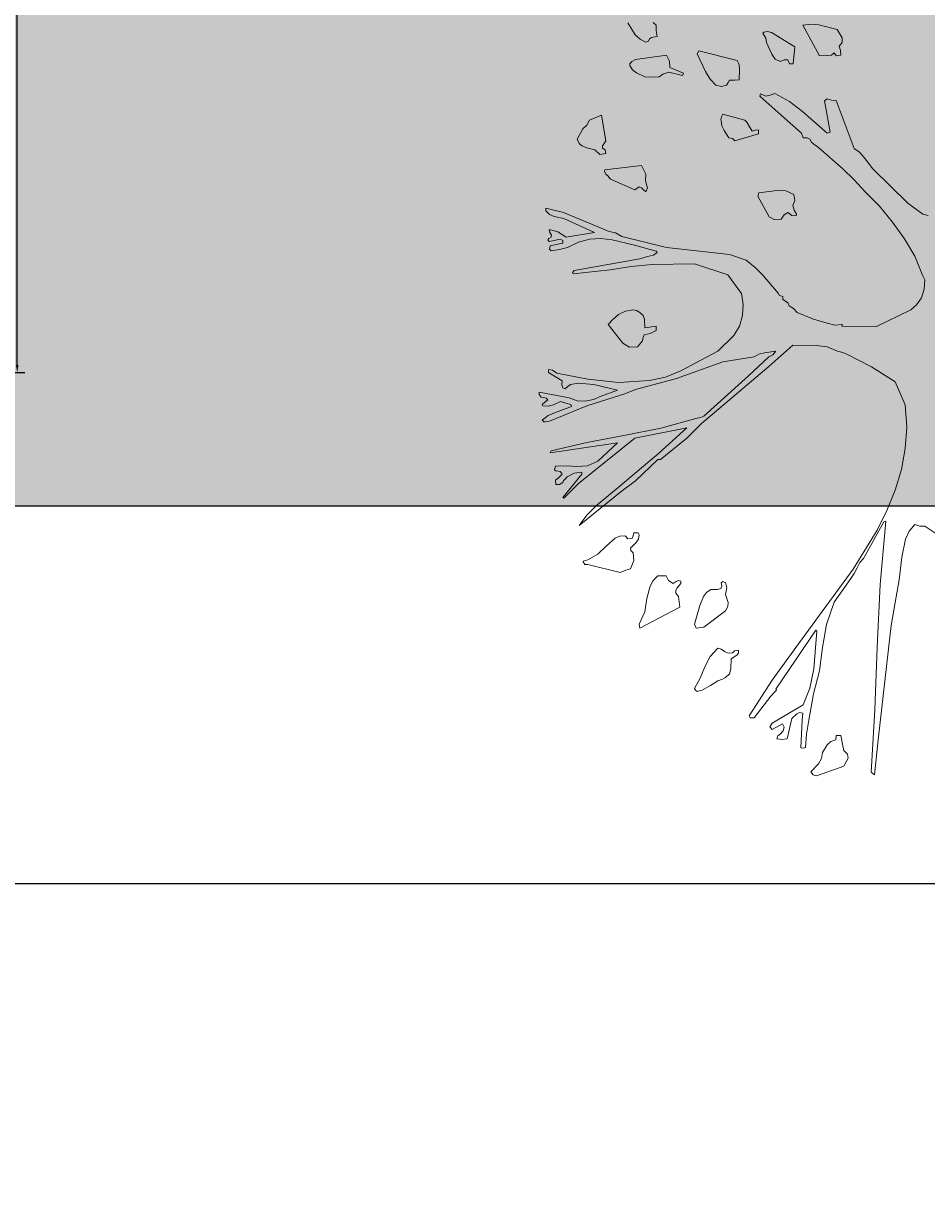
# Model space of a CAD drawing. Units: inches. Extents: x 84 to 1044, y -280 to 906.
# Tile 23 of 105: x 700 to 721, y -129 to -101. Entities that reach past the tile are written whole.
import ezdxf

# ---------------------------------------------------------------- set-up
doc = ezdxf.new("R2010")
doc.units = ezdxf.units.IN
for name, color, linetype, lineweight in [('A-ANNO-DIMS', 2, 'Continuous', 18), ('C-PROP', 7, 'Continuous', 25), ('L-PLNT', 114, 'Continuous', 15)]:
    doc.layers.add(name, color=color, linetype=linetype, lineweight=lineweight)
doc.layers.add('L-PLNT-PATT', color=9, linetype='Continuous', lineweight=9, true_color=0xafd9aa)
doc.styles.get("Standard").update_dxf_attribs({"font": 'arial.ttf'})
doc.dimstyles.get("Standard").update_dxf_attribs({"dimtxt": 0.18, "dimasz": 0.18, "dimexe": 0.18, "dimexo": 0.0625, "dimgap": 0.09, "dimtad": 0, "dimtih": 1, "dimtoh": 1, "dimdec": 4, "dimzin": 0, "dimdsep": 46, "dimtxsty": 'Standard', "dimcen": 0.09, "dimadec": 0, "dimazin": 0, "dimtfac": 1, "dimtdec": 4, "dimtofl": 0, "dimtmove": 0, "dimatfit": 3, "dimfxl": 1, "dimtolj": 1, "dimtzin": 0, "dimarcsym": 0})

# ---------------------------------------------------------------- blocks, each defined once
blk = doc.blocks.new('A$C37E508DF')
for p, q in [((0.1505, 1.189), (0.1389, 1.2079)), ((0.1784, 1.2083), (0.1831, 1.204)), ((0.1831, 1.204), (0.1831, 1.1959)), ((0.1831, 1.1959), (0.1848, 1.1865)), ((0.4134, 1.204), (0.4258, 1.2058)), ((0.4391, 1.156), (0.4134, 1.204)), ((0.4258, 1.2058), (0.4382, 1.2045)), ((0.4382, 1.2045), (0.4669, 1.1972)), ((0.4669, 1.1972), (0.4747, 1.1843)), ((0.1582, 1.1822), (0.1505, 1.189)), ((0.1668, 1.1775), (0.1582, 1.1822)), ((0.1711, 1.1792), (0.1668, 1.1775)), ((0.1728, 1.1826), (0.1711, 1.1792)), ((0.1758, 1.1847), (0.1728, 1.1826)), ((0.1788, 1.1852), (0.1758, 1.1847)), ((0.1848, 1.1865), (0.1788, 1.1852)), ((0.3507, 1.1916), (0.352, 1.1933)), ((0.355, 1.1839), (0.3507, 1.1916)), ((0.352, 1.1933), (0.3576, 1.1942)), ((0.3563, 1.177), (0.355, 1.1839)), ((0.3645, 1.1586), (0.3563, 1.177)), ((0.3576, 1.1942), (0.364, 1.1929)), ((0.364, 1.1929), (0.4005, 1.1702)), ((0.4751, 1.177), (0.47, 1.1714)), ((0.4747, 1.1843), (0.4751, 1.177)), ((0.2478, 1.1594), (0.2504, 1.1637)), ((0.2607, 1.1316), (0.2478, 1.1594)), ((0.2504, 1.1637), (0.3104, 1.1487)), ((0.37, 1.1509), (0.3645, 1.1586)), ((0.4005, 1.1702), (0.3979, 1.1436)), ((0.4622, 1.1607), (0.458, 1.1573)), ((0.4657, 1.156), (0.4622, 1.1607)), ((0.47, 1.1714), (0.4721, 1.1646)), ((0.4721, 1.1646), (0.473, 1.1573)), ((0.1419, 1.1436), (0.1449, 1.1474)), ((0.1419, 1.141), (0.1419, 1.1436)), ((0.1462, 1.1342), (0.1419, 1.141)), ((0.1449, 1.1474), (0.1509, 1.1504)), ((0.1509, 1.1504), (0.1994, 1.1573)), ((0.1994, 1.1573), (0.2041, 1.1479)), ((0.2041, 1.1479), (0.2045, 1.138)), ((0.3104, 1.1487), (0.3134, 1.1423)), ((0.3134, 1.1423), (0.3139, 1.1346)), ((0.3778, 1.1474), (0.37, 1.1509)), ((0.3842, 1.15), (0.3778, 1.1474)), ((0.3898, 1.15), (0.3842, 1.15)), ((0.3923, 1.1436), (0.3898, 1.15)), ((0.3979, 1.1436), (0.3923, 1.1436)), ((0.4519, 1.1564), (0.4391, 1.156)), ((0.458, 1.1573), (0.4519, 1.1564)), ((0.473, 1.1573), (0.4657, 1.156)), ((0.1522, 1.1294), (0.1462, 1.1342)), ((0.1655, 1.1234), (0.1522, 1.1294)), ((0.181, 1.1226), (0.1655, 1.1234)), ((0.1878, 1.1234), (0.181, 1.1226)), ((0.1938, 1.1273), (0.1878, 1.1234)), ((0.2032, 1.1303), (0.1938, 1.1273)), ((0.2247, 1.1251), (0.2032, 1.1303)), ((0.2045, 1.138), (0.226, 1.129)), ((0.226, 1.129), (0.2247, 1.1251)), ((0.268, 1.1196), (0.2607, 1.1316)), ((0.3139, 1.1346), (0.3134, 1.1183)), ((0.277, 1.1101), (0.268, 1.1196)), ((0.2856, 1.108), (0.277, 1.1101)), ((0.2933, 1.1101), (0.2856, 1.108)), ((0.2959, 1.1144), (0.2933, 1.1101)), ((0.2984, 1.1179), (0.2959, 1.1144)), ((0.3066, 1.1179), (0.2984, 1.1179)), ((0.3134, 1.1183), (0.3066, 1.1179)), ((0.3456, 1.093), (0.3469, 1.0964)), ((0.3842, 1.0591), (0.3456, 1.093)), ((0.3469, 1.0964), (0.355, 1.093)), ((0.355, 1.093), (0.3619, 1.0943)), ((0.3619, 1.0943), (0.3692, 1.0968)), ((0.3692, 1.0968), (0.3923, 1.0844)), ((0.4472, 1.0857), (0.4515, 1.0887)), ((0.4562, 1.0364), (0.4472, 1.0857)), ((0.4515, 1.0887), (0.4584, 1.0865)), ((0.4584, 1.0865), (0.4657, 1.0861)), ((0.4657, 1.0861), (0.4939, 1.0107)), ((0.3923, 1.0844), (0.4129, 1.069)), ((0.4129, 1.069), (0.4515, 1.0351)), ((0.0746, 1.0475), (0.0789, 1.0552)), ((0.0789, 1.0552), (0.0978, 1.063)), ((0.0978, 1.063), (0.1042, 1.0231)), ((0.2847, 1.0565), (0.2856, 1.0604)), ((0.2851, 1.054), (0.2847, 1.0565)), ((0.2864, 1.0463), (0.2851, 1.054)), ((0.2856, 1.0604), (0.2877, 1.0647)), ((0.2877, 1.0647), (0.3224, 1.0552)), ((0.3224, 1.0552), (0.3255, 1.0522)), ((0.3255, 1.0522), (0.3293, 1.0458)), ((0.4112, 1.0351), (0.3842, 1.0591)), ((0.0596, 1.0257), (0.0682, 1.0415)), ((0.0682, 1.0415), (0.0746, 1.0475)), ((0.2899, 1.039), (0.2864, 1.0463)), ((0.2972, 1.0274), (0.2899, 1.039)), ((0.3439, 1.0338), (0.3066, 1.0231)), ((0.3293, 1.0458), (0.3336, 1.0381)), ((0.3336, 1.0381), (0.3383, 1.0398)), ((0.3383, 1.0398), (0.3439, 1.0402)), ((0.3439, 1.0402), (0.3439, 1.0338)), ((0.4138, 1.0274), (0.4112, 1.0351)), ((0.4515, 1.0351), (0.4562, 1.0364)), ((0.0626, 1.0188), (0.0596, 1.0257)), ((0.0665, 1.0149), (0.0626, 1.0188)), ((0.0763, 1.0111), (0.0665, 1.0149)), ((0.1012, 1.018), (0.099, 1.0149)), ((0.099, 1.0149), (0.099, 1.0111)), ((0.1042, 1.0231), (0.1012, 1.018)), ((0.3032, 1.0265), (0.2972, 1.0274)), ((0.3066, 1.0231), (0.3032, 1.0265)), ((0.4202, 1.0274), (0.4138, 1.0274)), ((0.4241, 1.0257), (0.4202, 1.0274)), ((0.4267, 1.0209), (0.4241, 1.0257)), ((0.4305, 1.0175), (0.4267, 1.0209)), ((0.4378, 1.0124), (0.4305, 1.0175)), ((0.476, 0.9789), (0.4378, 1.0124)), ((0.087, 1.0085), (0.0763, 1.0111)), ((0.0948, 1.0016), (0.087, 1.0085)), ((0.1042, 1.0029), (0.0948, 1.0016)), ((0.099, 1.0111), (0.1033, 1.0085)), ((0.1033, 1.0085), (0.1042, 1.0029)), ((0.4939, 1.0107), (0.5021, 1.0051)), ((0.5021, 1.0051), (0.5094, 0.9969)), ((0.5094, 0.9969), (0.5231, 0.9789)), ((0.1025, 0.9751), (0.1029, 0.9772)), ((0.1046, 0.9708), (0.1025, 0.9751)), ((0.1029, 0.9772), (0.1604, 0.9841)), ((0.1604, 0.9841), (0.1672, 0.9708)), ((0.4939, 0.9618), (0.476, 0.9789)), ((0.5231, 0.9789), (0.578, 0.9253)), ((0.1076, 0.9682), (0.1046, 0.9708)), ((0.1119, 0.9626), (0.1076, 0.9682)), ((0.1496, 0.9463), (0.1119, 0.9626)), ((0.1672, 0.9708), (0.1664, 0.9601)), ((0.1664, 0.9601), (0.1698, 0.9493)), ((0.5111, 0.9429), (0.4939, 0.9618)), ((0.1565, 0.9506), (0.1496, 0.9463)), ((0.1604, 0.9493), (0.1565, 0.9506)), ((0.1629, 0.9468), (0.1604, 0.9493)), ((0.1672, 0.9429), (0.1629, 0.9468)), ((0.1698, 0.9493), (0.1672, 0.9429)), ((0.3426, 0.936), (0.3443, 0.9412)), ((0.3443, 0.9412), (0.3722, 0.9451)), ((0.3722, 0.9451), (0.3868, 0.9446)), ((0.3868, 0.9446), (0.3992, 0.9386)), ((0.3992, 0.9386), (0.4009, 0.9292)), ((0.5334, 0.9202), (0.5111, 0.9429)), ((0.3602, 0.9039), (0.3426, 0.936)), ((0.4009, 0.9292), (0.3975, 0.9215)), ((0.3975, 0.9215), (0.3996, 0.9142)), ((0.554, 0.8953), (0.5334, 0.9202)), ((0.578, 0.9253), (0.6011, 0.9077)), ((0.0103, 0.9129), (0.0103, 0.9172)), ((0.0103, 0.9172), (0.0382, 0.9107)), ((0.0159, 0.9073), (0.0103, 0.9129)), ((0.0232, 0.9043), (0.0159, 0.9073)), ((0.0386, 0.9013), (0.0232, 0.9043)), ((0.0382, 0.9107), (0.1098, 0.8807)), ((0.0866, 0.8794), (0.0386, 0.9013)), ((0.3692, 0.8992), (0.3602, 0.9039)), ((0.3838, 0.9069), (0.379, 0.9)), ((0.3898, 0.9107), (0.3838, 0.9069)), ((0.3958, 0.906), (0.3898, 0.9107)), ((0.4026, 0.9052), (0.3958, 0.906)), ((0.3996, 0.9142), (0.4031, 0.9077)), ((0.4031, 0.9077), (0.4026, 0.9052)), ((0.6011, 0.9077), (0.6097, 0.9056)), ((0.0159, 0.8803), (0.0154, 0.8837)), ((0.0154, 0.8837), (0.0292, 0.8803)), ((0.379, 0.9), (0.3692, 0.8992)), ((0.5728, 0.8691), (0.554, 0.8953)), ((0.0133, 0.8679), (0.015, 0.87)), ((0.0154, 0.8649), (0.0133, 0.8679)), ((0.015, 0.87), (0.0184, 0.8717)), ((0.0334, 0.8687), (0.0154, 0.8649)), ((0.0176, 0.8777), (0.0159, 0.8803)), ((0.0193, 0.8752), (0.0176, 0.8777)), ((0.0184, 0.8717), (0.0193, 0.8752)), ((0.0292, 0.8803), (0.0424, 0.8717)), ((0.0369, 0.8666), (0.0334, 0.8687)), ((0.0369, 0.8623), (0.0369, 0.8666)), ((0.0424, 0.8717), (0.0866, 0.8794)), ((0.0789, 0.8687), (0.0617, 0.864)), ((0.0965, 0.8696), (0.0789, 0.8687)), ((0.1141, 0.8679), (0.0965, 0.8696)), ((0.1098, 0.8807), (0.1196, 0.8786)), ((0.1492, 0.8593), (0.1141, 0.8679)), ((0.1196, 0.8786), (0.1295, 0.873)), ((0.1295, 0.873), (0.1994, 0.8554)), ((0.5887, 0.8421), (0.5728, 0.8691)), ((0.0163, 0.8529), (0.0171, 0.8584)), ((0.0184, 0.8503), (0.0163, 0.8529)), ((0.0171, 0.8584), (0.0266, 0.8602)), ((0.0317, 0.8524), (0.0184, 0.8503)), ((0.0266, 0.8602), (0.0369, 0.8623)), ((0.0442, 0.8554), (0.0317, 0.8524)), ((0.0617, 0.864), (0.0442, 0.8554)), ((0.1835, 0.8499), (0.1492, 0.8593)), ((0.1792, 0.8434), (0.1848, 0.8477)), ((0.1848, 0.8477), (0.1835, 0.8499)), ((0.1994, 0.8554), (0.2984, 0.8447)), ((0.0545, 0.8194), (0.1578, 0.8378)), ((0.1771, 0.8288), (0.1441, 0.8258)), ((0.1578, 0.8378), (0.1698, 0.8413)), ((0.1698, 0.8413), (0.1792, 0.8434)), ((0.2436, 0.8301), (0.1771, 0.8288)), ((0.2954, 0.813), (0.2436, 0.8301)), ((0.2984, 0.8447), (0.3242, 0.8357)), ((0.3242, 0.8357), (0.3387, 0.8241)), ((0.6007, 0.8125), (0.5887, 0.8421)), ((0.0519, 0.8164), (0.0545, 0.8194)), ((0.0532, 0.8143), (0.0519, 0.8164)), ((0.1111, 0.8207), (0.0532, 0.8143)), ((0.1441, 0.8258), (0.1111, 0.8207)), ((0.3173, 0.7834), (0.2954, 0.813)), ((0.3387, 0.8241), (0.3512, 0.8117)), ((0.3512, 0.8117), (0.3748, 0.7842)), ((0.6046, 0.8048), (0.6007, 0.8125)), ((0.6037, 0.7903), (0.6046, 0.8048)), ((0.3199, 0.7662), (0.3173, 0.7834)), ((0.3748, 0.7842), (0.3765, 0.7804)), ((0.3765, 0.7804), (0.3816, 0.7791)), ((0.3816, 0.7791), (0.382, 0.7744)), ((0.382, 0.7744), (0.3859, 0.7714)), ((0.5913, 0.7658), (0.599, 0.777)), ((0.599, 0.777), (0.6037, 0.7903)), ((0.1244, 0.7504), (0.1351, 0.7559)), ((0.1351, 0.7559), (0.1471, 0.7577)), ((0.1471, 0.7577), (0.1527, 0.7568)), ((0.1527, 0.7568), (0.1578, 0.7538)), ((0.3186, 0.7491), (0.3199, 0.7662)), ((0.3859, 0.7714), (0.3902, 0.7684)), ((0.3902, 0.7684), (0.3919, 0.7641)), ((0.3919, 0.7641), (0.3988, 0.7598)), ((0.3988, 0.7598), (0.4043, 0.7538)), ((0.5287, 0.7319), (0.5823, 0.7577)), ((0.5823, 0.7577), (0.5913, 0.7658)), ((0.1081, 0.7349), (0.1153, 0.7427)), ((0.1153, 0.7427), (0.1244, 0.7504)), ((0.1578, 0.7538), (0.1629, 0.7491)), ((0.1629, 0.7491), (0.1651, 0.7431)), ((0.1651, 0.7431), (0.1655, 0.7298)), ((0.3139, 0.7324), (0.3186, 0.7491)), ((0.4043, 0.7538), (0.4301, 0.7431)), ((0.4301, 0.7431), (0.4515, 0.7371)), ((0.4515, 0.7371), (0.4635, 0.7341)), ((0.1312, 0.7058), (0.1081, 0.7349)), ((0.1646, 0.7186), (0.1629, 0.7152)), ((0.1741, 0.7208), (0.1646, 0.7186)), ((0.1655, 0.7298), (0.1831, 0.7324)), ((0.1831, 0.7255), (0.1741, 0.7208)), ((0.1831, 0.7324), (0.1831, 0.7255)), ((0.28, 0.6933), (0.3049, 0.7178)), ((0.3049, 0.7178), (0.3139, 0.7324)), ((0.4635, 0.7341), (0.4755, 0.7349)), ((0.4755, 0.7349), (0.4742, 0.7324)), ((0.4742, 0.7324), (0.5287, 0.7319)), ((0.1415, 0.6994), (0.1312, 0.7058)), ((0.1539, 0.7002), (0.1415, 0.6994)), ((0.1621, 0.7092), (0.1539, 0.7002)), ((0.1629, 0.7152), (0.1621, 0.7092)), ((0.3975, 0.7028), (0.3598, 0.6693)), ((0.4339, 0.7019), (0.3975, 0.7028)), ((0.4515, 0.7002), (0.4339, 0.7019)), ((0.4674, 0.6933), (0.4515, 0.7002)), ((0.2221, 0.6625), (0.262, 0.6839)), ((0.262, 0.6839), (0.271, 0.6882)), ((0.271, 0.6882), (0.28, 0.6933)), ((0.337, 0.6843), (0.2877, 0.6762)), ((0.328, 0.6543), (0.3598, 0.6843)), ((0.3443, 0.6886), (0.337, 0.6843)), ((0.3533, 0.6903), (0.3443, 0.6886)), ((0.3709, 0.6933), (0.3533, 0.6903)), ((0.3598, 0.6843), (0.3662, 0.6873)), ((0.3662, 0.6873), (0.3709, 0.6933)), ((0.476, 0.6912), (0.4674, 0.6933)), ((0.4832, 0.6878), (0.476, 0.6912)), ((0.521, 0.6685), (0.4832, 0.6878)), ((0.0146, 0.6599), (0.0146, 0.6642)), ((0.0146, 0.6642), (0.0206, 0.6633)), ((0.0206, 0.6633), (0.0274, 0.6586)), ((0.1977, 0.6526), (0.2221, 0.6625)), ((0.2877, 0.6762), (0.2152, 0.6505)), ((0.3598, 0.6693), (0.2543, 0.5797)), ((0.5578, 0.6449), (0.521, 0.6685)), ((0.036, 0.6466), (0.0146, 0.6599)), ((0.0274, 0.6586), (0.0759, 0.6492)), ((0.0356, 0.6406), (0.036, 0.6466)), ((0.0759, 0.6492), (0.1244, 0.644)), ((0.1244, 0.644), (0.1728, 0.647)), ((0.2152, 0.6505), (0.1509, 0.6333)), ((0.1728, 0.647), (0.1977, 0.6526)), ((0.2581, 0.5913), (0.328, 0.6543)), ((0.5737, 0.6089), (0.5578, 0.6449)), ((0, 0.629), (0.0467, 0.62)), ((0, 0.6252), (0, 0.629)), ((0.0369, 0.6355), (0.0356, 0.6406)), ((0.0399, 0.6342), (0.0369, 0.6355)), ((0.0489, 0.641), (0.0399, 0.6342)), ((0.0609, 0.6428), (0.0489, 0.641)), ((0.0853, 0.641), (0.0609, 0.6428)), ((0.1226, 0.632), (0.0853, 0.641)), ((0.0973, 0.6226), (0.1226, 0.632)), ((0.1342, 0.6265), (0.1175, 0.6213)), ((0.1509, 0.6333), (0.1342, 0.6265)), ((0.003, 0.6213), (0, 0.6252)), ((0.0069, 0.6204), (0.003, 0.6213)), ((0.0047, 0.6093), (0.0086, 0.6132)), ((0.0056, 0.6076), (0.0047, 0.6093)), ((0.0141, 0.6072), (0.0056, 0.6076)), ((0.0107, 0.6196), (0.0069, 0.6204)), ((0.0086, 0.6132), (0.0133, 0.617)), ((0.0133, 0.617), (0.0107, 0.6196)), ((0.0223, 0.6089), (0.0141, 0.6072)), ((0.0746, 0.6076), (0.0163, 0.5836)), ((0.0334, 0.6145), (0.0223, 0.6089)), ((0.0416, 0.6119), (0.0334, 0.6145)), ((0.0493, 0.6093), (0.0416, 0.6119)), ((0.0467, 0.62), (0.0592, 0.6153)), ((0.0506, 0.6063), (0.0493, 0.6093)), ((0.0592, 0.6153), (0.072, 0.6149)), ((0.072, 0.6149), (0.0849, 0.6175)), ((0.1175, 0.6213), (0.0746, 0.6076)), ((0.0849, 0.6175), (0.0973, 0.6226)), ((0.5763, 0.5741), (0.5737, 0.6089)), ((0.0047, 0.5849), (0.0141, 0.5921)), ((0.0141, 0.5921), (0.0257, 0.5969)), ((0.0257, 0.5969), (0.0506, 0.6063)), ((0.2474, 0.5879), (0.253, 0.5892)), ((0.253, 0.5892), (0.2581, 0.5913)), ((0.0069, 0.5823), (0.0047, 0.5849)), ((0.0099, 0.5823), (0.0069, 0.5823)), ((0.0163, 0.5836), (0.0099, 0.5823)), ((0.1325, 0.5608), (0.1904, 0.5724)), ((0.2311, 0.5729), (0.1496, 0.557)), ((0.1869, 0.5325), (0.2311, 0.5729)), ((0.1904, 0.5724), (0.2474, 0.5879)), ((0.2543, 0.5797), (0.2311, 0.557)), ((0.5737, 0.5407), (0.5763, 0.5741)), ((0.1496, 0.557), (0.0613, 0.4858)), ((0.0746, 0.5501), (0.1325, 0.5608)), ((0.2311, 0.557), (0.1899, 0.5235)), ((0.1226, 0.5497), (0.0171, 0.5338)), ((0.0171, 0.5338), (0.0184, 0.5368)), ((0.0184, 0.5368), (0.0746, 0.5501)), ((0.0917, 0.5205), (0.1226, 0.5497)), ((0.5677, 0.5077), (0.5737, 0.5407)), ((0.0755, 0.5133), (0.0917, 0.5205)), ((0.1269, 0.482), (0.1869, 0.5325)), ((0.1861, 0.5231), (0.1509, 0.4897)), ((0.1899, 0.5235), (0.1861, 0.5231)), ((0.024, 0.5072), (0.0253, 0.5128)), ((0.0262, 0.5055), (0.024, 0.5072)), ((0.0253, 0.5128), (0.042, 0.5133)), ((0.0326, 0.5047), (0.0262, 0.5055)), ((0.03, 0.4948), (0.036, 0.5004)), ((0.036, 0.5004), (0.0326, 0.5047)), ((0.0369, 0.4639), (0.0669, 0.5004)), ((0.042, 0.5133), (0.0587, 0.5124)), ((0.0549, 0.5021), (0.0437, 0.4961)), ((0.0669, 0.5034), (0.0549, 0.5021)), ((0.0587, 0.5124), (0.0755, 0.5133)), ((0.0669, 0.5004), (0.0669, 0.5034)), ((0.5578, 0.4751), (0.5677, 0.5077)), ((0.0253, 0.491), (0.03, 0.4948)), ((0.0262, 0.4841), (0.0253, 0.491)), ((0.0317, 0.4841), (0.0262, 0.4841)), ((0.0369, 0.4871), (0.0317, 0.4841)), ((0.0382, 0.4905), (0.0369, 0.4871)), ((0.0403, 0.4922), (0.0382, 0.4905)), ((0.0613, 0.4858), (0.0386, 0.4627)), ((0.0437, 0.4961), (0.0403, 0.4922)), ((0.0905, 0.4515), (0.1269, 0.482)), ((0.1509, 0.4897), (0.1282, 0.4734)), ((0.0386, 0.4627), (0.0369, 0.4639)), ((0.1282, 0.4734), (0.0626, 0.4198)), ((0.545, 0.4434), (0.5578, 0.4751)), ((0.0746, 0.4361), (0.0905, 0.4515)), ((0.5295, 0.4125), (0.545, 0.4434)), ((0.0626, 0.4198), (0.0746, 0.4361)), ((0.5403, 0.4254), (0.5081, 0.3679)), ((0.5347, 0.3276), (0.5433, 0.4266)), ((0.5433, 0.4266), (0.5403, 0.4254)), ((0.1471, 0.4035), (0.1484, 0.4082)), ((0.1484, 0.4082), (0.1548, 0.4082)), ((0.1548, 0.4082), (0.1565, 0.4052)), ((0.1565, 0.4052), (0.1556, 0.3983)), ((0.4922, 0.3516), (0.5295, 0.4125)), ((0.5797, 0.4112), (0.5741, 0.3983)), ((0.5887, 0.4215), (0.5797, 0.4112)), ((0.5969, 0.4189), (0.5887, 0.4215)), ((0.6046, 0.4189), (0.5969, 0.4189)), ((0.6295, 0.4022), (0.6046, 0.4189)), ((0.0917, 0.3748), (0.1055, 0.388)), ((0.1055, 0.388), (0.1192, 0.4001)), ((0.1192, 0.4001), (0.1265, 0.4031)), ((0.1265, 0.4031), (0.1346, 0.4039)), ((0.1346, 0.4039), (0.1389, 0.3992)), ((0.1389, 0.3992), (0.1458, 0.3996)), ((0.1518, 0.3932), (0.1432, 0.3842)), ((0.1458, 0.3996), (0.1471, 0.4035)), ((0.1556, 0.3983), (0.1518, 0.3932)), ((0.5741, 0.3983), (0.5686, 0.3705)), ((0.0763, 0.3662), (0.0917, 0.3748)), ((0.1432, 0.3842), (0.1436, 0.3808)), ((0.1436, 0.3808), (0.1471, 0.3769)), ((0.1471, 0.3769), (0.1484, 0.3649)), ((0.5081, 0.3679), (0.5025, 0.3619)), ((0.5686, 0.3705), (0.5643, 0.3349)), ((0.069, 0.364), (0.0763, 0.3662)), ((0.069, 0.3627), (0.069, 0.364)), ((0.0716, 0.3585), (0.069, 0.3627)), ((0.0763, 0.3585), (0.0716, 0.3585)), ((0.1269, 0.3464), (0.0763, 0.3585)), ((0.1355, 0.3499), (0.1269, 0.3464)), ((0.1432, 0.352), (0.1355, 0.3499)), ((0.1484, 0.3649), (0.1432, 0.352)), ((0.4065, 0.2345), (0.4922, 0.3516)), ((0.4982, 0.3537), (0.4939, 0.3447)), ((0.5025, 0.3619), (0.4982, 0.3537)), ((0.1737, 0.325), (0.1788, 0.3336)), ((0.1788, 0.3336), (0.1861, 0.3409)), ((0.1861, 0.3409), (0.199, 0.3409)), ((0.199, 0.3409), (0.2024, 0.3336)), ((0.2024, 0.3336), (0.2097, 0.3289)), ((0.2097, 0.3289), (0.2148, 0.3323)), ((0.2148, 0.3323), (0.2182, 0.3336)), ((0.2182, 0.3336), (0.2221, 0.3327)), ((0.2221, 0.3327), (0.2221, 0.3289)), ((0.2851, 0.3302), (0.2877, 0.3319)), ((0.2877, 0.3319), (0.292, 0.3306)), ((0.4884, 0.337), (0.4622, 0.2997)), ((0.4939, 0.3447), (0.4884, 0.337)), ((0.5643, 0.3349), (0.5578, 0.2993)), ((0.1689, 0.3053), (0.1737, 0.325)), ((0.2161, 0.3224), (0.214, 0.3186)), ((0.214, 0.3186), (0.214, 0.3139)), ((0.214, 0.3139), (0.2182, 0.3087)), ((0.2221, 0.3289), (0.2161, 0.3224)), ((0.2577, 0.3087), (0.2624, 0.3147)), ((0.2624, 0.3147), (0.2689, 0.3194)), ((0.2689, 0.3194), (0.2796, 0.3194)), ((0.2796, 0.3194), (0.2847, 0.3211)), ((0.2847, 0.3211), (0.2864, 0.325)), ((0.2864, 0.325), (0.2851, 0.3302)), ((0.292, 0.3306), (0.2941, 0.322)), ((0.2941, 0.322), (0.292, 0.3117)), ((0.53, 0.229), (0.5347, 0.3276)), ((0.1655, 0.2843), (0.1689, 0.3053)), ((0.2182, 0.3087), (0.2204, 0.292)), ((0.2436, 0.265), (0.2517, 0.2946)), ((0.2517, 0.2946), (0.2577, 0.3087)), ((0.292, 0.3117), (0.2959, 0.2993)), ((0.2959, 0.2993), (0.2954, 0.2928)), ((0.4622, 0.2997), (0.4502, 0.2645)), ((0.5578, 0.2993), (0.5518, 0.2633)), ((0.1565, 0.265), (0.1655, 0.2843)), ((0.2204, 0.292), (0.1578, 0.259)), ((0.292, 0.286), (0.2581, 0.2607)), ((0.2954, 0.2928), (0.292, 0.286)), ((0.1578, 0.259), (0.1565, 0.265)), ((0.2461, 0.259), (0.2436, 0.265)), ((0.2581, 0.2607), (0.2461, 0.259)), ((0.4502, 0.2645), (0.4438, 0.2285)), ((0.5518, 0.2633), (0.5475, 0.2268)), ((0.4335, 0.2556), (0.3709, 0.1634)), ((0.4305, 0.1951), (0.4352, 0.2543)), ((0.4352, 0.2543), (0.4335, 0.2556)), ((0.268, 0.2148), (0.28, 0.2277)), ((0.28, 0.2277), (0.2851, 0.226)), ((0.2851, 0.226), (0.2903, 0.2225)), ((0.2903, 0.2225), (0.2963, 0.22)), ((0.3027, 0.2204), (0.3061, 0.2234)), ((0.3061, 0.2234), (0.3122, 0.2247)), ((0.3122, 0.2247), (0.3122, 0.22)), ((0.3649, 0.1775), (0.4065, 0.2345)), ((0.4438, 0.2285), (0.4391, 0.1921)), ((0.5261, 0.1308), (0.53, 0.229)), ((0.5475, 0.2268), (0.5313, 0.084)), ((0.2594, 0.1981), (0.268, 0.2148)), ((0.2963, 0.22), (0.3027, 0.2204)), ((0.301, 0.211), (0.3002, 0.1951)), ((0.3096, 0.2165), (0.301, 0.211)), ((0.3122, 0.22), (0.3096, 0.2165)), ((0.2521, 0.1805), (0.2594, 0.1981)), ((0.298, 0.1874), (0.292, 0.1818)), ((0.3002, 0.1951), (0.298, 0.1874)), ((0.4241, 0.1651), (0.4305, 0.1951)), ((0.4391, 0.1921), (0.4301, 0.1561)), ((0.2436, 0.1642), (0.2521, 0.1805)), ((0.2684, 0.1689), (0.2556, 0.1616)), ((0.28, 0.1762), (0.2684, 0.1689)), ((0.2873, 0.1788), (0.28, 0.1762)), ((0.292, 0.1818), (0.2873, 0.1788)), ((0.3293, 0.1213), (0.3649, 0.1775)), ((0.2448, 0.1616), (0.2436, 0.1642)), ((0.2478, 0.1599), (0.2448, 0.1616)), ((0.2508, 0.1608), (0.2478, 0.1599)), ((0.2556, 0.1616), (0.2508, 0.1608)), ((0.3628, 0.1526), (0.337, 0.1183)), ((0.3692, 0.1591), (0.3628, 0.1526)), ((0.3718, 0.1616), (0.3692, 0.1591)), ((0.3709, 0.1634), (0.3718, 0.1616)), ((0.4138, 0.1389), (0.4241, 0.1651)), ((0.4301, 0.1561), (0.4224, 0.1145)), ((0.3653, 0.1098), (0.4138, 0.1389)), ((0.5205, 0.033), (0.5261, 0.1308)), ((0.3306, 0.1183), (0.3293, 0.1213)), ((0.337, 0.1183), (0.3306, 0.1183)), ((0.3962, 0.1175), (0.3885, 0.0853)), ((0.4039, 0.1248), (0.3962, 0.1175)), ((0.4082, 0.1269), (0.4039, 0.1248)), ((0.4134, 0.1256), (0.4082, 0.1269)), ((0.4099, 0.0716), (0.4121, 0.1145)), ((0.4121, 0.1145), (0.4134, 0.1256)), ((0.4224, 0.1145), (0.4189, 0.093)), ((0.3615, 0.1042), (0.3653, 0.1098)), ((0.3653, 0.0999), (0.3615, 0.1042)), ((0.3812, 0.1089), (0.3653, 0.0999)), ((0.3739, 0.09), (0.3782, 0.0935)), ((0.3782, 0.0935), (0.3825, 0.0978)), ((0.3842, 0.1037), (0.3812, 0.1089)), ((0.3825, 0.0978), (0.3842, 0.1037)), ((0.4189, 0.093), (0.4176, 0.072)), ((0.3722, 0.0853), (0.3739, 0.09)), ((0.3808, 0.0845), (0.3722, 0.0853)), ((0.3885, 0.0853), (0.3808, 0.0845)), ((0.4442, 0.0639), (0.4515, 0.0763)), ((0.4515, 0.0763), (0.4571, 0.0815)), ((0.4571, 0.0815), (0.4648, 0.084)), ((0.4648, 0.084), (0.4657, 0.0905)), ((0.4657, 0.0905), (0.473, 0.0905)), ((0.473, 0.0905), (0.476, 0.0746)), ((0.476, 0.0746), (0.4777, 0.0673)), ((0.5313, 0.084), (0.5257, 0.0291)), ((0.4142, 0.0707), (0.4099, 0.0716)), ((0.4176, 0.072), (0.4142, 0.0707)), ((0.4425, 0.0544), (0.4442, 0.0639)), ((0.4777, 0.0673), (0.4832, 0.0613)), ((0.4845, 0.0553), (0.4811, 0.0493)), ((0.4832, 0.0613), (0.4845, 0.0553)), ((0.4258, 0.0339), (0.4378, 0.0463)), ((0.4777, 0.0424), (0.4348, 0.0274)), ((0.4378, 0.0463), (0.4425, 0.0544)), ((0.4811, 0.0493), (0.4777, 0.0424)), ((0.4296, 0.0291), (0.4258, 0.0339)), ((0.4348, 0.0274), (0.4296, 0.0291)), ((0.5257, 0.0291), (0.5205, 0.033))]:
    blk.add_line(p, q)
blk = doc.blocks.new('*D30')
at = {"layer": 'A-ANNO-DIMS', "color": 0, "lineweight": -2, "transparency": 16777216}
for p, q in [((696.303, -86.54), (699.895, -86.54)), ((699.715, -86.72), (699.715, -97.938)), ((699.715, -109.523), (699.715, -98.305)), ((696.303, -109.703), (699.895, -109.703))]:
    blk.add_line(p, q, dxfattribs=at)
at = {"layer": 'A-ANNO-DIMS', "color": 0, "transparency": 16777216}
for points in [[(699.685, -86.72), (699.745, -86.72), (699.715, -86.54)], [(699.685, -109.523), (699.745, -109.523), (699.715, -109.703)]]:
    blk.add_solid(points, dxfattribs=at)
at = {"layer": 'Defpoints', "color": 0, "transparency": 16777216}
for p in [(696.24, -86.54), (699.715, -86.54), (696.24, -109.703)]:
    blk.add_point(p, dxfattribs=at)
at = {"layer": 'A-ANNO-DIMS', "color": 0, "transparency": 16777216, "insert": (699.715, -98.121), "char_height": 0.18, "attachment_point": 5}
blk.add_mtext('\\A1;SHRUB 23 TYP.', dxfattribs=at)
blk = doc.blocks.new('*D60')
at = {"layer": 'A-ANNO-DIMS', "color": 0, "lineweight": -2, "transparency": 16777216}
for p, q in [((134.179, -121.942), (134.179, -180.64)), ((992.074, -121.942), (992.074, -180.64)), ((134.359, -180.46), (562.733, -180.46)), ((991.894, -180.46), (563.521, -180.46))]:
    blk.add_line(p, q, dxfattribs=at)
at = {"layer": 'A-ANNO-DIMS', "color": 0, "transparency": 16777216}
for points in [[(134.359, -180.43), (134.359, -180.49), (134.179, -180.46)], [(991.894, -180.43), (991.894, -180.49), (992.074, -180.46)]]:
    blk.add_solid(points, dxfattribs=at)
at = {"layer": 'Defpoints', "color": 0, "transparency": 16777216}
for p in [(134.179, -121.88), (992.074, -121.88), (992.074, -180.46)]:
    blk.add_point(p, dxfattribs=at)
at = {"layer": 'A-ANNO-DIMS', "color": 0, "transparency": 16777216, "insert": (563.127, -180.46), "char_height": 0.18, "attachment_point": 5}
blk.add_mtext('\\A1;857.9', dxfattribs=at)

msp = doc.modelspace()

# ---------------------------------------------------------------- hatches: boundary and pattern name
at = {"layer": 'L-PLNT-PATT', "transparency": 33554597}
h = msp.add_hatch(color=256, dxfattribs=at)
h.dxf.hatch_style = 1
h.paths.add_polyline_path([(791.074, 31.12), (791.074, 91.12), (743.074, 91.12), (674.074, 91.12), (674.074, 31.12), (650.074, 31.12), (650.074, -112.88), (983.074, -112.88), (983.074, -64.88), (791.074, -64.88)])

# ---------------------------------------------------------------- linework, layer by layer
at = {"layer": 'C-PROP'}
for points in [[(143.179, -121.88), (134.179, -121.88), (134.179, 856.12), (992.074, 856.12), (992.074, -121.88), (624.574, -121.88)], [(143.179, -112.88), (143.179, 847.12), (983.074, 847.12), (983.074, -112.88), (624.574, -112.88)]]:
    msp.add_lwpolyline(points, dxfattribs=at)

# ---------------------------------------------------------------- block references
at = {"layer": 'L-PLNT', "xscale": 15.19586232982809, "yscale": 15.19586232982809, "zscale": 15.19586232982809}
msp.add_blockref('A$C37E508DF', (712.152, -119.725, 0), dxfattribs=at)

# ---------------------------------------------------------------- dimensions: what is measured, and where the dimension line sits
at = {"layer": 'A-ANNO-DIMS'}
dim = msp.add_linear_dim(base=(699.715, -86.54), p1=(696.24, -109.703), p2=(696.24, -86.54), angle=90, text='SHRUB <> TYP.', dimstyle='Standard', override={"dimdec": 0, "dimlfac": 1, "dimrnd": 0, "dimzin": 0, "dimdsep": 46, "dimlunit": 2}, dxfattribs=at)
dim.commit()
dim.dimension.update_dxf_attribs({"geometry": '*D30', "text_midpoint": (699.715, -98.121)})
dim = msp.add_linear_dim(base=(992.074, -180.46), p1=(134.179, -121.88), p2=(992.074, -121.88), dimstyle='Standard', override={"dimdec": 1, "dimlfac": 1, "dimrnd": 0, "dimzin": 0, "dimdsep": 46, "dimlunit": 2}, dxfattribs=at)
dim.commit()
dim.dimension.update_dxf_attribs({"geometry": '*D60', "text_midpoint": (563.127, -180.46)})

doc.saveas('drawing.dxf')
